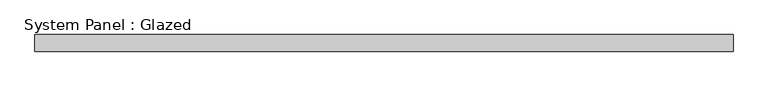
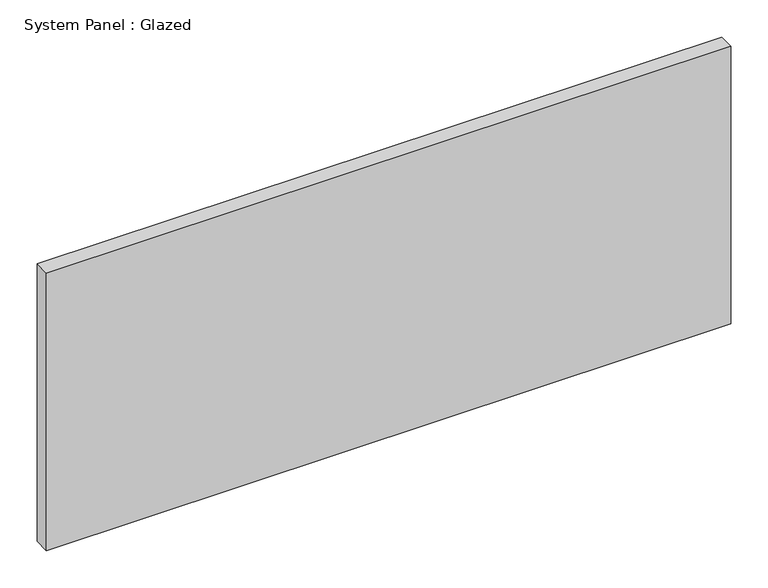
"""IFC4 building model written with IfcOpenShell, lengths in millimetres: plate geometry, System Panel : Glazed."""

from ifc_helpers import new_model, si_unit, origin, origin_with_axes, place, context, project, spatial, polyline, outline, extrude, source, transform, mapped, element, save


def system_panel_glazed_20ce4246(model_context):
    return source(origin(), model_context, "Body", "SweptSolid", [
        extrude(outline(polyline([(533.3999998, -44.45), (-533.3999998, -44.45), (-533.3999998, -19.05), (533.3999998, -19.05), (533.3999998, -44.45)])), origin_with_axes(), (0.0, 0.0, 1.0), 457.2),
    ])


if __name__ == "__main__":
    model = new_model("IFC4")
    model_context = context("Model", 3, world=origin())
    ifc_project = project(units=[si_unit("LENGTHUNIT", "METRE", prefix="MILLI")], contexts=[model_context])
    site = spatial("IfcSite", under=ifc_project)
    building = spatial("IfcBuilding", under=site)
    placement = place(None, origin())
    system_panel_glazed_shape = system_panel_glazed_20ce4246(model_context)
    element("IfcPlate", 1, ObjectType="System Panel : Glazed", at=placement, inside=building, context=model_context, shape_type="MappedRepresentation", body=[
        mapped(system_panel_glazed_shape, transform((0.0, 0.0, 0.0), x_axis=(1.0, 0.0, 0.0), y_axis=(0.0, 1.0, 0.0), z_axis=(0.0, 0.0, 1.0))),
    ])
    save(model, "model.ifc")

# Revit data of these elements
# Type "System Panel : Glazed"
#   Construction Type Id = "GSP4R"
#   Analytic Construction = "1/8 in Pilkington single glazing"
#   Visual Light Transmittance = 0.9
#   Solar Heat Gain Coefficient = 0.86
#   Heat Transfer Coefficient (U) = 1.18115 BTU/(h·ft²·°F)
#   Define Thermal Properties by = 1
# Element 1 (IfcPlate, "System Panel : Glazed")
#   Materials on its faces: "Glass"
# Materials
#   "Glass": class "Glass", colour RGB 0 128 192, transparency 0.75, Description = "Soda Lime Glass", Cost = 0
